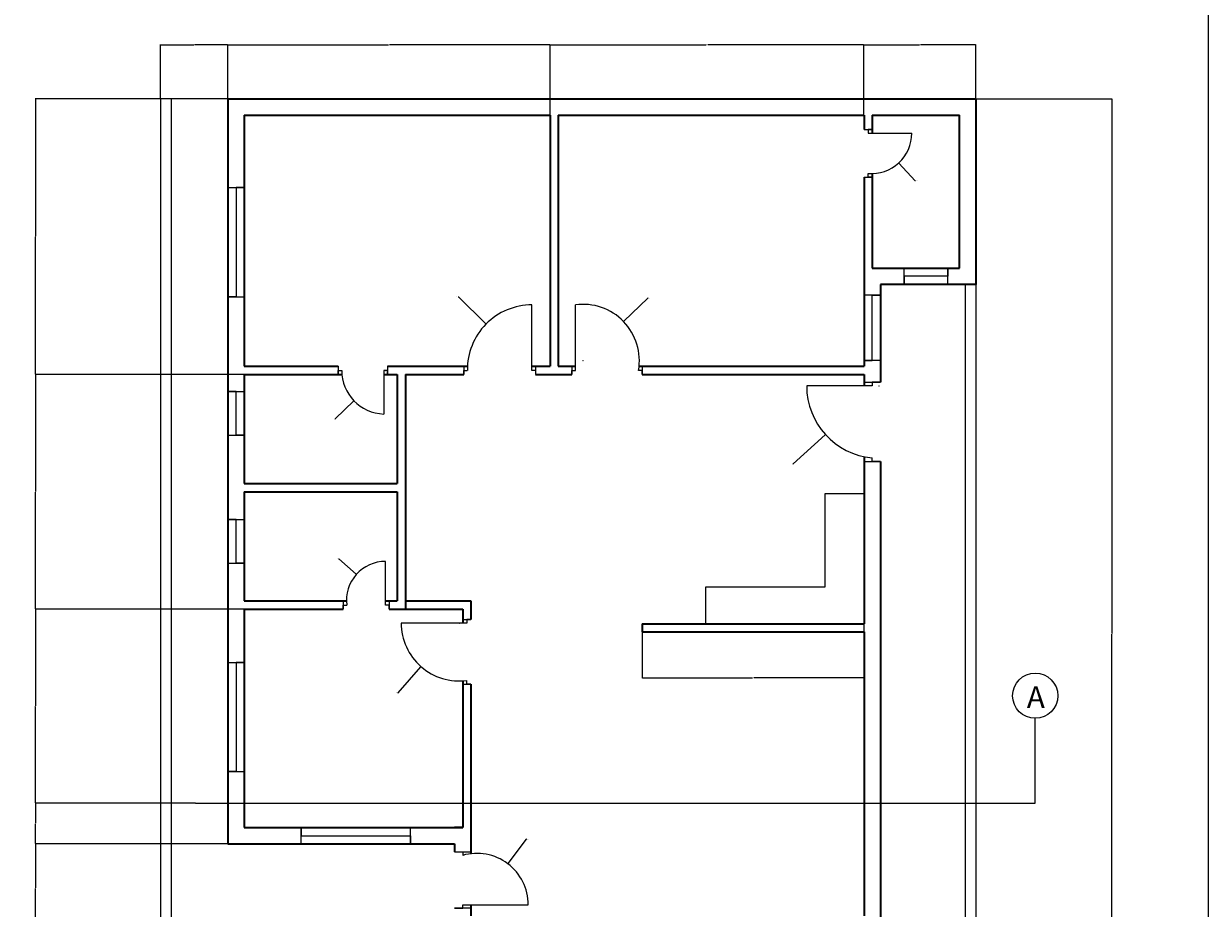
# Model space of a CAD drawing. Units: inches. Extents: x 1587 to 2880, y 1287 to 2423.
# Tile 7 of 8: x 2229 to 2880, y 1543 to 2030. Entities that reach past the tile are written whole.
import ezdxf

# ---------------------------------------------------------------- set-up
doc = ezdxf.new("R2010")
doc.units = ezdxf.units.IN
for name, color, linetype, lineweight in [('A-ANNO-DIMS', 2, 'Continuous', 18), ('A-ANNO-SYMB', 5, 'Continuous', 25), ('A-ANNO-TTLB', 7, 'Continuous', 25), ('A-DOOR', 3, 'Continuous', 18), ('A-FLOR-FIXT', 8, 'Continuous', 18), ('A-GLAZ', 4, 'Continuous', 18), ('A-WALL', 7, 'Continuous', 35), ('C-PROP', 8, 'Continuous', 25)]:
    doc.layers.add(name, color=color, linetype=linetype, lineweight=lineweight)
doc.layers.add('A-WALL-PATT', color=251, linetype='Continuous', lineweight=13, true_color=0x636466)
doc.styles.get("Standard").update_dxf_attribs({"font": 'arial.ttf'})
doc.dimstyles.get("Standard").update_dxf_attribs({"dimtxt": 0.18, "dimasz": 0.18, "dimexe": 0.18, "dimexo": 0.0625, "dimgap": 0.09, "dimtad": 0, "dimtih": 1, "dimtoh": 1, "dimdec": 4, "dimzin": 0, "dimdsep": 46, "dimtxsty": 'Standard', "dimcen": 0.09, "dimadec": 0, "dimazin": 0, "dimtfac": 1, "dimtdec": 4, "dimtofl": 0, "dimtmove": 0, "dimatfit": 3, "dimfxl": 1, "dimtolj": 1, "dimtzin": 0, "dimarcsym": 0})

# ---------------------------------------------------------------- blocks, each defined once
blk = doc.blocks.new('WIN-60IN')
for p, q in [((0, 60), (9, 60)), ((9, 60), (4.5, 60)), ((4.5, 60), (4.5, 0)), ((4.5, 0), (0, 0)), ((0, 0), (9, 0))]:
    blk.add_line(p, q)
blk = doc.blocks.new('WIN-24IN')
for p, q in [((0, 9), (0, 0)), ((24, 4.5), (24, 9)), ((24, 9), (24, 0)), ((0, 0), (0, 4.5)), ((0, 4.5), (24, 4.5))]:
    blk.add_line(p, q)
blk = doc.blocks.new('WIN-36IN')
for p, q in [((0, 36), (9, 36)), ((9, 36), (4.5, 36)), ((4.5, 36), (4.5, 0)), ((4.5, 0), (0, 0)), ((0, 0), (9, 0))]:
    blk.add_line(p, q)
blk = doc.blocks.new('DOOR-24IN-GUEST-BATH')
for p, q in [((23.33, 2.25), (23.33, 26.25)), ((0, 4.5), (0, 0)), ((0, 0), (0, 2.25)), ((0, 2.25), (2, 2.25)), ((25.33, 2.25), (23.33, 2.25)), ((25.33, 4.5), (25.33, 0)), ((25.33, 0), (25.33, 2.25))]:
    blk.add_line(p, q)
blk.add_arc((23.33, 4.77), 21.48, 90, 186.73236)
blk = doc.blocks.new('DOOR-24IN-BED1-BATH')
for p, q in [((0, 26.25), (0, 21.75)), ((27.11, 26.25), (27.11, 21.75)), ((0, 21.75), (0, 24)), ((0, 24), (2, 24)), ((27.11, 24), (25.11, 24)), ((25.11, 24), (25.11, 0)), ((27.11, 21.75), (27.11, 24))]:
    blk.add_line(p, q)
blk.add_arc((26.02, 24), 24.02, 180, 267.83008)
blk = doc.blocks.new('DOOR-36IN-BED1')
for p, q in [((37.52, 2.25), (37.52, 38.25)), ((0, 4.5), (0, 0)), ((0, 0), (0, 2.25)), ((0, 2.25), (2, 2.25)), ((39.52, 2.25), (37.52, 2.25)), ((39.52, 4.5), (39.52, 0))]:
    blk.add_line(p, q)
blk.add_arc((37.52, 2.73), 35.52, 90, 180.77456)
blk = doc.blocks.new('DOOR-36IN-BED2')
for p, q in [((2, 2.25), (2, 38.25)), ((0, 4.5), (0, 0)), ((0, 0), (0, 2.25)), ((0, 2.25), (2, 2.25)), ((38.7, 2.25), (36.7, 2.25)), ((38.7, 4.5), (38.7, 0)), ((38.7, 0), (38.7, 2.25))]:
    blk.add_line(p, q)
blk.add_arc((6.24, 7.62), 30.93, 350.00897, 97.87967)
blk = doc.blocks.new('DOOR-24IN-BED2-BATH')
for p, q in [((0, 26.03), (4.5, 26.03)), ((4.5, 26.03), (2.25, 26.03)), ((2.25, 26.03), (2.25, 24.03)), ((2.25, 24.03), (26.25, 24.03)), ((0, 0), (4.5, 0)), ((2.25, 0), (2.25, 2)), ((4.5, 0), (2.25, 0))]:
    blk.add_line(p, q)
blk.add_arc((4.13, 24.03), 22.12, 265.1111, 0)
blk = doc.blocks.new('DOOR-36IN-ENTRY')
for p, q in [((0, 31.08), (9, 31.08)), ((4.5, 31.08), (4.5, 29.08)), ((9, 0), (0, 0)), ((0, 0), (4.5, 0)), ((4.5, 0), (4.5, 2)), ((4.5, 2), (40.5, 2))]:
    blk.add_line(p, q)
blk.add_arc((12.32, 2), 28.18, 0, 106.09946)
blk = doc.blocks.new('DOOR-36IN-GUEST')
for p, q in [((36, 33.56), (0, 33.56)), ((33.75, 35.56), (38.25, 35.56)), ((38.25, 35.56), (36, 35.56)), ((36, 35.56), (36, 33.56)), ((33.75, 0), (38.25, 0)), ((36, 0), (36, 2)), ((38.25, 0), (36, 0))]:
    blk.add_line(p, q)
blk.add_arc((31.83, 33.56), 31.83, 180, 277.524)
blk = doc.blocks.new('DOOR-36IN-KITCHEN')
for p, q in [((36, 41.64), (0, 41.64)), ((31.5, 43.64), (31.5, 43.64)), ((31.5, 43.64), (40.5, 43.64)), ((40.5, 43.64), (36, 43.64)), ((36, 43.64), (36, 41.64)), ((31.5, 0), (40.5, 0)), ((36, 0), (36, 2)), ((40.5, 0), (36, 0))]:
    blk.add_line(p, q)
blk.add_arc((39.83, 41.64), 39.83, 180, 264.48319)
blk = doc.blocks.new('COUNTER-L-PLAN')
for p, q in [((65.63, 20.29), (65.63, 71.6)), ((65.63, 71.6), (86.95, 71.6)), ((0, 0), (0, 20.29)), ((0, 20.29), (65.63, 20.29))]:
    blk.add_line(p, q)
blk = doc.blocks.new('*D46')
at = {"layer": 'A-ANNO-DIMS', "color": 0, "lineweight": -2, "transparency": 16777216}
for p, q in [((2752.6, 1988.39), (2827.47, 1988.39)), ((2827.29, 1988.21), (2827.29, 1694.57)), ((2827.29, 1400.57), (2827.29, 1694.2)), ((2752.6, 1400.39), (2827.47, 1400.39))]:
    blk.add_line(p, q, dxfattribs=at)
at = {"layer": 'A-ANNO-DIMS', "color": 0, "transparency": 16777216}
for points in [[(2827.26, 1988.21), (2827.32, 1988.21), (2827.29, 1988.39)], [(2827.26, 1400.57), (2827.32, 1400.57), (2827.29, 1400.39)]]:
    blk.add_solid(points, dxfattribs=at)
at = {"layer": 'Defpoints', "color": 0, "transparency": 16777216}
for p in [(2752.53, 1988.39), (2827.29, 1988.39), (2752.53, 1400.39)]:
    blk.add_point(p, dxfattribs=at)
at = {"layer": 'A-ANNO-DIMS', "color": 0, "transparency": 16777216, "insert": (2827.29, 1694.39), "char_height": 0.18, "attachment_point": 5}
blk.add_mtext('\\A1;588', dxfattribs=at)
blk = doc.blocks.new('*D48')
at = {"layer": 'A-ANNO-DIMS', "color": 0, "lineweight": -2, "transparency": 16777216}
for p, q in [((2304.53, 1988.45), (2304.53, 2018.32)), ((2304.71, 2018.14), (2322.82, 2018.14)), ((2341.35, 2018.14), (2323.25, 2018.14)), ((2341.53, 1988.45), (2341.53, 2018.32))]:
    blk.add_line(p, q, dxfattribs=at)
at = {"layer": 'A-ANNO-DIMS', "color": 0, "transparency": 16777216}
for points in [[(2304.71, 2018.17), (2304.71, 2018.11), (2304.53, 2018.14)], [(2341.35, 2018.17), (2341.35, 2018.11), (2341.53, 2018.14)]]:
    blk.add_solid(points, dxfattribs=at)
at = {"layer": 'Defpoints', "color": 0, "transparency": 16777216}
for p in [(2341.53, 2018.14), (2304.53, 1988.39), (2341.53, 1988.39)]:
    blk.add_point(p, dxfattribs=at)
at = {"layer": 'A-ANNO-DIMS', "color": 0, "transparency": 16777216, "insert": (2323.03, 2018.14), "char_height": 0.18, "attachment_point": 5}
blk.add_mtext('\\A1;37', dxfattribs=at)
blk = doc.blocks.new('*D49')
at = {"layer": 'A-ANNO-DIMS', "color": 0, "lineweight": -2, "transparency": 16777216}
for p, q in [((2341.53, 1988.45), (2341.53, 2018.32)), ((2341.71, 2018.14), (2429.75, 2018.14)), ((2518.35, 2018.14), (2430.31, 2018.14)), ((2518.53, 1979.45), (2518.53, 2018.32))]:
    blk.add_line(p, q, dxfattribs=at)
at = {"layer": 'A-ANNO-DIMS', "color": 0, "transparency": 16777216}
for points in [[(2341.71, 2018.17), (2341.71, 2018.11), (2341.53, 2018.14)], [(2518.35, 2018.17), (2518.35, 2018.11), (2518.53, 2018.14)]]:
    blk.add_solid(points, dxfattribs=at)
at = {"layer": 'Defpoints', "color": 0, "transparency": 16777216}
for p in [(2518.53, 2018.14), (2341.53, 1988.39), (2518.53, 1979.39)]:
    blk.add_point(p, dxfattribs=at)
at = {"layer": 'A-ANNO-DIMS', "color": 0, "transparency": 16777216, "insert": (2430.03, 2018.14), "char_height": 0.18, "attachment_point": 5}
blk.add_mtext('\\A1;177', dxfattribs=at)
blk = doc.blocks.new('*D50')
at = {"layer": 'A-ANNO-DIMS', "color": 0, "lineweight": -2, "transparency": 16777216}
for p, q in [((2518.53, 1979.45), (2518.53, 2018.32)), ((2518.71, 2018.14), (2604.4, 2018.14)), ((2690.85, 2018.14), (2605.17, 2018.14)), ((2691.03, 1979.45), (2691.03, 2018.32))]:
    blk.add_line(p, q, dxfattribs=at)
at = {"layer": 'A-ANNO-DIMS', "color": 0, "transparency": 16777216}
for points in [[(2518.71, 2018.17), (2518.71, 2018.11), (2518.53, 2018.14)], [(2690.85, 2018.17), (2690.85, 2018.11), (2691.03, 2018.14)]]:
    blk.add_solid(points, dxfattribs=at)
at = {"layer": 'Defpoints', "color": 0, "transparency": 16777216}
for p in [(2691.03, 2018.14), (2518.53, 1979.39), (2691.03, 1979.39)]:
    blk.add_point(p, dxfattribs=at)
at = {"layer": 'A-ANNO-DIMS', "color": 0, "transparency": 16777216, "insert": (2604.78, 2018.14), "char_height": 0.18, "attachment_point": 5}
blk.add_mtext('\\A1;172.5', dxfattribs=at)
blk = doc.blocks.new('*D51')
at = {"layer": 'A-ANNO-DIMS', "color": 0, "lineweight": -2, "transparency": 16777216}
for p, q in [((2691.03, 1979.45), (2691.03, 2018.32)), ((2691.21, 2018.14), (2721.46, 2018.14)), ((2752.35, 2018.14), (2722.11, 2018.14)), ((2752.53, 1988.45), (2752.53, 2018.32))]:
    blk.add_line(p, q, dxfattribs=at)
at = {"layer": 'A-ANNO-DIMS', "color": 0, "transparency": 16777216}
for points in [[(2691.21, 2018.17), (2691.21, 2018.11), (2691.03, 2018.14)], [(2752.35, 2018.17), (2752.35, 2018.11), (2752.53, 2018.14)]]:
    blk.add_solid(points, dxfattribs=at)
at = {"layer": 'Defpoints', "color": 0, "transparency": 16777216}
for p in [(2752.53, 2018.14), (2752.53, 1988.39), (2691.03, 1979.39)]:
    blk.add_point(p, dxfattribs=at)
at = {"layer": 'A-ANNO-DIMS', "color": 0, "transparency": 16777216, "insert": (2721.78, 2018.14), "char_height": 0.18, "attachment_point": 5}
blk.add_mtext('\\A1;61.5', dxfattribs=at)
blk = doc.blocks.new('*D58')
at = {"layer": 'A-ANNO-DIMS', "color": 0, "lineweight": -2, "transparency": 16777216}
for p, q in [((2341.47, 1578.89), (2235.59, 1578.89)), ((2235.77, 1578.71), (2235.77, 1554.82)), ((2235.77, 1530.57), (2235.77, 1554.45)), ((2465.97, 1530.39), (2235.59, 1530.39))]:
    blk.add_line(p, q, dxfattribs=at)
at = {"layer": 'A-ANNO-DIMS', "color": 0, "transparency": 16777216}
for points in [[(2235.74, 1578.71), (2235.8, 1578.71), (2235.77, 1578.89)], [(2235.74, 1530.57), (2235.8, 1530.57), (2235.77, 1530.39)]]:
    blk.add_solid(points, dxfattribs=at)
at = {"layer": 'Defpoints', "color": 0, "transparency": 16777216}
for p in [(2235.77, 1578.89), (2341.53, 1578.89), (2466.03, 1530.39)]:
    blk.add_point(p, dxfattribs=at)
at = {"layer": 'A-ANNO-DIMS', "color": 0, "transparency": 16777216, "insert": (2235.77, 1554.64), "char_height": 0.18, "attachment_point": 5}
blk.add_mtext('\\A1;48.5', dxfattribs=at)
blk = doc.blocks.new('*D59')
at = {"layer": 'A-ANNO-DIMS', "color": 0, "lineweight": -2, "transparency": 16777216}
for p, q in [((2265.45, 1601.25), (2235.59, 1601.25)), ((2235.77, 1601.07), (2235.77, 1590.25)), ((2235.77, 1579.07), (2235.77, 1589.88)), ((2341.47, 1578.89), (2235.59, 1578.89))]:
    blk.add_line(p, q, dxfattribs=at)
at = {"layer": 'A-ANNO-DIMS', "color": 0, "transparency": 16777216}
for points in [[(2235.74, 1601.07), (2235.8, 1601.07), (2235.77, 1601.25)], [(2235.74, 1579.07), (2235.8, 1579.07), (2235.77, 1578.89)]]:
    blk.add_solid(points, dxfattribs=at)
at = {"layer": 'Defpoints', "color": 0, "transparency": 16777216}
for p in [(2235.77, 1601.25), (2265.52, 1601.25), (2341.53, 1578.89)]:
    blk.add_point(p, dxfattribs=at)
at = {"layer": 'A-ANNO-DIMS', "color": 0, "transparency": 16777216, "insert": (2235.77, 1590.07), "char_height": 0.18, "attachment_point": 5}
blk.add_mtext('\\A1;22.36', dxfattribs=at)
blk = doc.blocks.new('*D60')
at = {"layer": 'A-ANNO-DIMS', "color": 0, "lineweight": -2, "transparency": 16777216}
for p, q in [((2350.47, 1707.89), (2235.59, 1707.89)), ((2235.77, 1707.71), (2235.77, 1654.75)), ((2235.77, 1601.43), (2235.77, 1654.38)), ((2265.45, 1601.25), (2235.59, 1601.25))]:
    blk.add_line(p, q, dxfattribs=at)
at = {"layer": 'A-ANNO-DIMS', "color": 0, "transparency": 16777216}
for points in [[(2235.74, 1707.71), (2235.8, 1707.71), (2235.77, 1707.89)], [(2235.74, 1601.43), (2235.8, 1601.43), (2235.77, 1601.25)]]:
    blk.add_solid(points, dxfattribs=at)
at = {"layer": 'Defpoints', "color": 0, "transparency": 16777216}
for p in [(2235.77, 1707.89), (2350.53, 1707.89), (2265.52, 1601.25)]:
    blk.add_point(p, dxfattribs=at)
at = {"layer": 'A-ANNO-DIMS', "color": 0, "transparency": 16777216, "insert": (2235.77, 1654.57), "char_height": 0.18, "attachment_point": 5}
blk.add_mtext('\\A1;106.64', dxfattribs=at)
blk = doc.blocks.new('*D61')
at = {"layer": 'A-ANNO-DIMS', "color": 0, "lineweight": -2, "transparency": 16777216}
for p, q in [((2350.47, 1836.89), (2235.59, 1836.89)), ((2235.77, 1836.71), (2235.77, 1772.57)), ((2235.77, 1708.07), (2235.77, 1772.2)), ((2350.47, 1707.89), (2235.59, 1707.89))]:
    blk.add_line(p, q, dxfattribs=at)
at = {"layer": 'A-ANNO-DIMS', "color": 0, "transparency": 16777216}
for points in [[(2235.74, 1836.71), (2235.8, 1836.71), (2235.77, 1836.89)], [(2235.74, 1708.07), (2235.8, 1708.07), (2235.77, 1707.89)]]:
    blk.add_solid(points, dxfattribs=at)
at = {"layer": 'Defpoints', "color": 0, "transparency": 16777216}
for p in [(2235.77, 1836.89), (2350.53, 1836.89), (2350.53, 1707.89)]:
    blk.add_point(p, dxfattribs=at)
at = {"layer": 'A-ANNO-DIMS', "color": 0, "transparency": 16777216, "insert": (2235.77, 1772.39), "char_height": 0.18, "attachment_point": 5}
blk.add_mtext('\\A1;129', dxfattribs=at)
blk = doc.blocks.new('*D62')
at = {"layer": 'A-ANNO-DIMS', "color": 0, "lineweight": -2, "transparency": 16777216}
for p, q in [((2341.47, 1988.39), (2235.59, 1988.39)), ((2235.77, 1988.21), (2235.77, 1912.82)), ((2235.77, 1837.07), (2235.77, 1912.45)), ((2350.47, 1836.89), (2235.59, 1836.89))]:
    blk.add_line(p, q, dxfattribs=at)
at = {"layer": 'A-ANNO-DIMS', "color": 0, "transparency": 16777216}
for points in [[(2235.74, 1988.21), (2235.8, 1988.21), (2235.77, 1988.39)], [(2235.74, 1837.07), (2235.8, 1837.07), (2235.77, 1836.89)]]:
    blk.add_solid(points, dxfattribs=at)
at = {"layer": 'Defpoints', "color": 0, "transparency": 16777216}
for p in [(2235.77, 1988.39), (2341.53, 1988.39), (2350.53, 1836.89)]:
    blk.add_point(p, dxfattribs=at)
at = {"layer": 'A-ANNO-DIMS', "color": 0, "transparency": 16777216, "insert": (2235.77, 1912.64), "char_height": 0.18, "attachment_point": 5}
blk.add_mtext('\\A1;151.5', dxfattribs=at)
blk = doc.blocks.new('*D81')
at = {"layer": 'A-ANNO-DIMS', "color": 0, "lineweight": -2, "transparency": 16777216}
for p, q in [((2569.14, 1699.82), (2569.14, 1669.96)), ((2691.03, 1699.82), (2691.03, 1669.96)), ((2569.32, 1670.14), (2629.7, 1670.14)), ((2690.85, 1670.14), (2630.47, 1670.14))]:
    blk.add_line(p, q, dxfattribs=at)
at = {"layer": 'A-ANNO-DIMS', "color": 0, "transparency": 16777216}
for points in [[(2569.32, 1670.17), (2569.32, 1670.11), (2569.14, 1670.14)], [(2690.85, 1670.17), (2690.85, 1670.11), (2691.03, 1670.14)]]:
    blk.add_solid(points, dxfattribs=at)
at = {"layer": 'Defpoints', "color": 0, "transparency": 16777216}
for p in [(2569.14, 1699.89), (2691.03, 1699.89), (2569.14, 1670.14)]:
    blk.add_point(p, dxfattribs=at)
at = {"layer": 'A-ANNO-DIMS', "color": 0, "transparency": 16777216, "insert": (2630.09, 1670.14), "char_height": 0.18, "attachment_point": 5}
blk.add_mtext('\\A1;121.9', dxfattribs=at)
blk = doc.blocks.new('*D100')
at = {"layer": 'A-ANNO-DIMS', "color": 0, "lineweight": -2, "transparency": 16777216}
for p, q in [((2699.27, 1830.63), (2699.45, 1830.63)), ((2699.36, 1830.54), (2699.36, 1830.72)), ((2652.18, 1787.79), (2669.74, 1803.74)), ((2652, 1787.79), (2652.18, 1787.79))]:
    blk.add_line(p, q, dxfattribs=at)
at = {"layer": 'A-ANNO-DIMS', "color": 0, "transparency": 16777216}
blk.add_solid([(2669.72, 1803.76), (2669.76, 1803.71), (2669.88, 1803.86)], dxfattribs=at)
at = {"layer": 'Defpoints', "color": 0, "transparency": 16777216}
for p in [(2699.36, 1830.63), (2669.88, 1803.86)]:
    blk.add_point(p, dxfattribs=at)
at = {"layer": 'A-ANNO-DIMS', "color": 0, "transparency": 16777216, "insert": (2651.53, 1787.79), "char_height": 0.18, "attachment_point": 5}
blk.add_mtext('\\A1;R39.83', dxfattribs=at)
blk = doc.blocks.new('*D101')
at = {"layer": 'A-ANNO-DIMS', "color": 0, "lineweight": -2, "transparency": 16777216}
for p, q in [((2467.97, 1879.53), (2468.15, 1879.53)), ((2468.15, 1879.53), (2483.2, 1864.69)), ((2508.52, 1839.62), (2508.7, 1839.62)), ((2508.61, 1839.53), (2508.61, 1839.71))]:
    blk.add_line(p, q, dxfattribs=at)
at = {"layer": 'A-ANNO-DIMS', "color": 0, "transparency": 16777216}
blk.add_solid([(2483.22, 1864.71), (2483.17, 1864.67), (2483.32, 1864.56)], dxfattribs=at)
at = {"layer": 'Defpoints', "color": 0, "transparency": 16777216}
for p in [(2483.32, 1864.56), (2508.61, 1839.62)]:
    blk.add_point(p, dxfattribs=at)
at = {"layer": 'A-ANNO-DIMS', "color": 0, "transparency": 16777216, "insert": (2467.49, 1879.53), "char_height": 0.18, "attachment_point": 5}
blk.add_mtext('\\A1;R35.52', dxfattribs=at)
blk = doc.blocks.new('*D102')
at = {"layer": 'A-ANNO-DIMS', "color": 0, "lineweight": -2, "transparency": 16777216}
for p, q in [((2468.53, 1700.27), (2468.71, 1700.27)), ((2468.62, 1700.18), (2468.62, 1700.36)), ((2435.04, 1661.97), (2447.51, 1676.2)), ((2434.86, 1661.97), (2435.04, 1661.97))]:
    blk.add_line(p, q, dxfattribs=at)
at = {"layer": 'A-ANNO-DIMS', "color": 0, "transparency": 16777216}
blk.add_solid([(2447.49, 1676.22), (2447.54, 1676.18), (2447.63, 1676.33)], dxfattribs=at)
at = {"layer": 'Defpoints', "color": 0, "transparency": 16777216}
for p in [(2468.62, 1700.27), (2447.63, 1676.33)]:
    blk.add_point(p, dxfattribs=at)
at = {"layer": 'A-ANNO-DIMS', "color": 0, "transparency": 16777216, "insert": (2434.38, 1661.97), "char_height": 0.18, "attachment_point": 5}
blk.add_mtext('\\A1;R31.83', dxfattribs=at)
blk = doc.blocks.new('*D103')
at = {"layer": 'A-ANNO-DIMS', "color": 0, "lineweight": -2, "transparency": 16777216}
for p, q in [((2572.32, 1878.84), (2559.08, 1866.09)), ((2572.5, 1878.84), (2572.32, 1878.84)), ((2536.6, 1844.5), (2536.78, 1844.5)), ((2536.69, 1844.41), (2536.69, 1844.59))]:
    blk.add_line(p, q, dxfattribs=at)
at = {"layer": 'A-ANNO-DIMS', "color": 0, "transparency": 16777216}
blk.add_solid([(2559.06, 1866.11), (2559.11, 1866.07), (2558.96, 1865.96)], dxfattribs=at)
at = {"layer": 'Defpoints', "color": 0, "transparency": 16777216}
for p in [(2558.96, 1865.96), (2536.69, 1844.5)]:
    blk.add_point(p, dxfattribs=at)
at = {"layer": 'A-ANNO-DIMS', "color": 0, "transparency": 16777216, "insert": (2573.05, 1878.84), "char_height": 0.18, "attachment_point": 5}
blk.add_mtext('\\A1;R30.926', dxfattribs=at)
blk = doc.blocks.new('*D104')
at = {"layer": 'A-ANNO-DIMS', "color": 0, "lineweight": -2, "transparency": 16777216}
for p, q in [((2505.46, 1581.52), (2495.4, 1568.15)), ((2505.64, 1581.52), (2505.46, 1581.52)), ((2478.26, 1545.48), (2478.44, 1545.48)), ((2478.35, 1545.39), (2478.35, 1545.57))]:
    blk.add_line(p, q, dxfattribs=at)
at = {"layer": 'A-ANNO-DIMS', "color": 0, "transparency": 16777216}
blk.add_solid([(2495.38, 1568.16), (2495.42, 1568.13), (2495.29, 1568)], dxfattribs=at)
at = {"layer": 'Defpoints', "color": 0, "transparency": 16777216}
for p in [(2495.29, 1568), (2478.35, 1545.48)]:
    blk.add_point(p, dxfattribs=at)
at = {"layer": 'A-ANNO-DIMS', "color": 0, "transparency": 16777216, "insert": (2506.19, 1581.52), "char_height": 0.18, "attachment_point": 5}
blk.add_mtext('\\A1;R28.184', dxfattribs=at)
blk = doc.blocks.new('*D105')
at = {"layer": 'A-ANNO-DIMS', "color": 0, "lineweight": -2, "transparency": 16777216}
for p, q in [((2428.01, 1839.14), (2428.19, 1839.14)), ((2428.1, 1839.05), (2428.1, 1839.23)), ((2400.42, 1812.48), (2410.67, 1822.35)), ((2400.24, 1812.48), (2400.42, 1812.48))]:
    blk.add_line(p, q, dxfattribs=at)
at = {"layer": 'A-ANNO-DIMS', "color": 0, "transparency": 16777216}
blk.add_solid([(2410.65, 1822.38), (2410.69, 1822.33), (2410.8, 1822.48)], dxfattribs=at)
at = {"layer": 'Defpoints', "color": 0, "transparency": 16777216}
for p in [(2428.1, 1839.14), (2410.8, 1822.48)]:
    blk.add_point(p, dxfattribs=at)
at = {"layer": 'A-ANNO-DIMS', "color": 0, "transparency": 16777216, "insert": (2399.69, 1812.48), "char_height": 0.18, "attachment_point": 5}
blk.add_mtext('\\A1;R24.017', dxfattribs=at)
blk = doc.blocks.new('*D106')
at = {"layer": 'A-ANNO-DIMS', "color": 0, "lineweight": -2, "transparency": 16777216}
for p, q in [((2695.08, 1969.44), (2695.26, 1969.44)), ((2695.17, 1969.35), (2695.17, 1969.53)), ((2719.1, 1943.37), (2710.25, 1953.02)), ((2719.28, 1943.37), (2719.1, 1943.37))]:
    blk.add_line(p, q, dxfattribs=at)
at = {"layer": 'A-ANNO-DIMS', "color": 0, "transparency": 16777216}
blk.add_solid([(2710.27, 1953.04), (2710.22, 1953), (2710.13, 1953.15)], dxfattribs=at)
at = {"layer": 'Defpoints', "color": 0, "transparency": 16777216}
for p in [(2695.17, 1969.44), (2710.13, 1953.15)]:
    blk.add_point(p, dxfattribs=at)
at = {"layer": 'A-ANNO-DIMS', "color": 0, "transparency": 16777216, "insert": (2719.83, 1943.37), "char_height": 0.18, "attachment_point": 5}
blk.add_mtext('\\A1;R22.115', dxfattribs=at)
blk = doc.blocks.new('*D107')
at = {"layer": 'A-ANNO-DIMS', "color": 0, "lineweight": -2, "transparency": 16777216}
for p, q in [((2402.28, 1735.49), (2402.46, 1735.49)), ((2402.46, 1735.49), (2411.96, 1727.05)), ((2428.06, 1712.66), (2428.24, 1712.66)), ((2428.15, 1712.57), (2428.15, 1712.75))]:
    blk.add_line(p, q, dxfattribs=at)
at = {"layer": 'A-ANNO-DIMS', "color": 0, "transparency": 16777216}
blk.add_solid([(2411.98, 1727.07), (2411.94, 1727.02), (2412.09, 1726.93)], dxfattribs=at)
at = {"layer": 'Defpoints', "color": 0, "transparency": 16777216}
for p in [(2412.09, 1726.93), (2428.15, 1712.66)]:
    blk.add_point(p, dxfattribs=at)
at = {"layer": 'A-ANNO-DIMS', "color": 0, "transparency": 16777216, "insert": (2401.8, 1735.49), "char_height": 0.18, "attachment_point": 5}
blk.add_mtext('\\A1;R21.48', dxfattribs=at)

msp = doc.modelspace()

# ---------------------------------------------------------------- hatches: boundary and pattern name
at = {"layer": 'A-WALL-PATT'}
h = msp.add_hatch(color=256, dxfattribs=at)
h.dxf.hatch_style = 1
h.paths.add_polyline_path([(2190.3423, 1988.3868), (2181.3423, 1988.3868), (2137.8423, 1988.3868), (1779.3423, 1988.3868), (1779.3423, 1939.6287), (1788.3423, 1939.6287), (1788.3423, 1979.3868), (1956.3423, 1979.3868), (1956.3423, 1841.3868), (1948.4175, 1841.3868), (1948.4175, 1836.8868), (1968.256, 1836.8868), (1968.256, 1839.1368), (1968.256, 1841.3868), (1960.8423, 1841.3868), (1960.8423, 1979.3868), (2128.8423, 1979.3868), (2128.8423, 1971.4394), (2133.3423, 1971.4394), (2133.3423, 1979.3868), (2181.3423, 1979.3868), (2181.3423, 1895.3868), (2174.9842, 1895.3868), (2174.9842, 1886.3868), (2190.3423, 1886.3868), (2190.3423, 1895.3868)])
h.paths.add_polyline_path([(1788.3423, 1879.6287), (1779.3423, 1879.6287), (1779.3423, 1827.4437), (1788.3423, 1827.4437), (1788.3423, 1836.8868), (1839.8915, 1836.8868), (1839.8915, 1839.1368), (1839.8915, 1841.3868), (1788.3423, 1841.3868)])
h.paths.add_polyline_path([(1876.8423, 1836.8868), (1908.901, 1836.8868), (1908.901, 1839.1368), (1908.901, 1841.3868), (1866.9993, 1841.3868), (1866.9993, 1836.8868), (1872.3423, 1836.8868), (1872.3423, 1776.8868), (1788.3423, 1776.8868), (1788.3423, 1803.4437), (1779.3423, 1803.4437), (1779.3423, 1757.1447), (1788.3423, 1757.1447), (1788.3423, 1772.3868), (1872.3423, 1772.3868), (1872.3423, 1712.3868), (1867.9542, 1712.3868), (1867.9542, 1707.8868), (1876.8423, 1707.8868), (1876.8423, 1772.3868)])
h.paths.add_polyline_path([(1842.6206, 1710.1368), (1842.6206, 1712.3868), (1788.3423, 1712.3868), (1788.3423, 1733.1447), (1779.3423, 1733.1447), (1779.3423, 1678.6557), (1788.3423, 1678.6557), (1788.3423, 1707.8868), (1842.6206, 1707.8868)])
h.paths.add_polyline_path([(1912.8423, 1712.3868), (1908.3423, 1712.3868), (1876.8423, 1712.3868), (1876.8423, 1707.8868), (1908.3423, 1707.8868), (1908.3423, 1702.2679), (1912.8423, 1702.2679)])
h.paths.add_polyline_path([(2137.8423, 1844.5168), (2128.8423, 1844.5168), (2128.8423, 1841.3868), (2006.9533, 1841.3868), (2006.9533, 1836.8868), (2128.8423, 1836.8868), (2128.8423, 1832.632), (2137.8423, 1832.632)])
h.paths.add_polyline_path([(1997.6598, 1534.8868), (1997.6598, 1539.3868), (1912.8423, 1539.3868), (1912.8423, 1543.4794), (1903.8423, 1543.4794), (1903.8423, 1530.3868), (1997.6598, 1530.3868)])
h.paths.add_polyline_path([(1912.8423, 1666.7101), (1910.5923, 1666.7101), (1908.3423, 1666.7101), (1908.3423, 1587.8868), (1903.8423, 1587.8868), (1879.6624, 1587.8868), (1879.6624, 1578.8868), (1903.8423, 1578.8868), (1903.8423, 1574.5584), (1912.8423, 1574.5584), (1912.8423, 1578.8868), (1912.8423, 1587.8868)])
h.paths.add_polyline_path([(1788.3423, 1618.6557), (1779.3423, 1618.6557), (1779.3423, 1578.8868), (1819.6624, 1578.8868), (1819.6624, 1583.3868), (1819.6624, 1587.8868), (1788.3423, 1587.8868)])
h.paths.add_polyline_path([(2133.3423, 1945.4046), (2131.0923, 1945.4046), (2128.8423, 1945.4046), (2128.8423, 1880.5168), (2137.8423, 1880.5168), (2137.8423, 1886.3868), (2150.9842, 1886.3868), (2150.9842, 1890.8868), (2150.9842, 1895.3868), (2133.3423, 1895.3868)], flags=17)
h.paths.add_polyline_path([(2137.8423, 1788.9874), (2133.3423, 1788.9874), (2128.8423, 1788.9874), (2128.8423, 1699.8868), (2006.9533, 1699.8868), (2006.9533, 1695.3868), (2128.8423, 1695.3868), (2128.8423, 1539.3868), (2057.6598, 1539.3868), (2057.6598, 1530.3868), (2128.8423, 1530.3868), (2128.8423, 1461.3868), (1988.2941, 1461.3868), (1988.2941, 1452.3868), (2137.8423, 1452.3868), (2137.8423, 1530.3868)])
h.paths.add_polyline_path([(1866.9166, 1348.94), (2042.3313, 1348.94), (2042.3313, 1371.6078), (1866.9166, 1371.6078)], flags=9)
h.paths.add_polyline_path([(2758.0473, 2126.4845), (2848.522, 2126.4845), (2848.522, 2138.8487), (2758.0473, 2138.8487)], flags=9)
h.paths.add_polyline_path([(2742.9428, 2216.0014), (2782.483, 2216.0014), (2782.483, 2228.3657), (2742.9428, 2228.3657)], flags=9)
h.paths.add_polyline_path([(2749.234, 2261.9992), (2784.0963, 2261.9992), (2784.0963, 2274.3634), (2749.234, 2274.3634)], flags=9)
h.paths.add_polyline_path([(2733.8012, 2281.8262), (2817.7726, 2281.8262), (2817.7726, 2294.1904), (2733.8012, 2294.1904)], flags=9)
h.paths.add_polyline_path([(2422.857, 2073.081), (2531.34, 2073.081), (2531.34, 2097.8095), (2422.857, 2097.8095)], flags=9)
h.paths.add_polyline_path([(1856.7732, 2082.3109), (1956.866, 2082.3109), (1956.866, 2107.0394), (1856.7732, 2107.0394)], flags=9)
h.paths.add_polyline_path([(2777.4581, 1646.9437), (2794.6887, 1646.9437), (2794.6887, 1671.6723), (2777.4581, 1671.6723)], flags=9)
h.paths.add_polyline_path([(2585.5416, 1728.5169), (2655.2006, 1728.5169), (2655.2006, 1760.9057), (2585.5416, 1760.9057)], flags=9)
h.paths.add_polyline_path([(2554.1301, 1617.6432), (2608.2079, 1617.6432), (2608.2079, 1640.032), (2554.1301, 1640.032)], flags=9)
h.paths.add_polyline_path([(2359.8658, 1678.1191), (2437.8454, 1678.1191), (2437.8454, 1700.5079), (2359.8658, 1700.5079)], flags=9)
h.paths.add_polyline_path([(2392.0171, 1749.26), (2422.3411, 1749.26), (2422.3411, 1767.9173), (2392.0171, 1767.9173)], flags=9)
h.paths.add_polyline_path([(2391.9937, 1787.5799), (2422.3177, 1787.5799), (2422.3177, 1806.2373), (2391.9937, 1806.2373)], flags=9)
h.paths.add_polyline_path([(2707.7632, 1927.6903), (2738.1623, 1927.6903), (2738.1623, 1946.3477), (2707.7632, 1946.3477)], flags=9)
h.paths.add_polyline_path([(2581.5534, 1846.9887), (2635.6148, 1846.9887), (2635.6148, 1869.3775), (2581.5534, 1869.3775)], flags=9)
h.paths.add_polyline_path([(2382.3802, 1864.4978), (2436.4416, 1864.4978), (2436.4416, 1886.8866), (2382.3802, 1886.8866)], flags=9)
h.paths.add_polyline_path([(2023.35, 1728.5169), (2093.0089, 1728.5169), (2093.0089, 1760.9057), (2023.35, 1760.9057)], flags=25)
h.paths.add_polyline_path([(1991.9385, 1617.6432), (2046.0162, 1617.6432), (2046.0162, 1640.032), (1991.9385, 1640.032)], flags=25)
h.paths.add_polyline_path([(1791.1103, 1678.1191), (1869.0899, 1678.1191), (1869.0899, 1700.5079), (1791.1103, 1700.5079)], flags=9)
h.paths.add_polyline_path([(1829.8255, 1749.26), (1860.1495, 1749.26), (1860.1495, 1767.9173), (1829.8255, 1767.9173)], flags=25)
h.paths.add_polyline_path([(1829.8021, 1787.5799), (1860.1261, 1787.5799), (1860.1261, 1806.2373), (1829.8021, 1806.2373)], flags=25)
h.paths.add_polyline_path([(2145.5716, 1927.6903), (2175.9706, 1927.6903), (2175.9706, 1946.3477), (2145.5716, 1946.3477)], flags=25)
h.paths.add_polyline_path([(2019.3617, 1846.9887), (2073.4231, 1846.9887), (2073.4231, 1869.3775), (2019.3617, 1869.3775)], flags=25)
h.paths.add_polyline_path([(1820.1886, 1864.4978), (1874.25, 1864.4978), (1874.25, 1886.8866), (1820.1886, 1886.8866)], flags=25)

# ---------------------------------------------------------------- linework, layer by layer
at = {"layer": 'A-ANNO-SYMB'}
for p, q in [((2785.1198, 1601.2461), (2785.1198, 1647.901)), ((2323.7941, 1601.2461), (2265.516, 1601.2461)), ((2323.7941, 1601.2461), (2785.1198, 1601.2461))]:
    msp.add_line(p, q, dxfattribs=at)
msp.add_circle((2785.1198, 1660.3223), 12.4213, dxfattribs=at)
at = {"layer": 'A-ANNO-TTLB'}
msp.add_lwpolyline([(1586.5185, 2423.1539), (2880.2062, 2423.1539), (2880.2062, 1286.9347), (1586.5185, 1286.9347)], close=True, dxfattribs=at)
at = {"layer": 'A-WALL'}
for p, q in [((2341.534, 1988.3868), (2341.534, 1578.8868)), ((2341.534, 1988.3868), (2341.534, 1578.8868)), ((2341.534, 1988.3868), (2700.034, 1988.3868)), ((2691.034, 1988.3868), (2695.534, 1988.3868)), ((2700.034, 1988.3868), (2748.034, 1988.3868)), ((2743.534, 1988.3868), (2752.534, 1988.3868)), ((2752.534, 1988.3868), (2752.534, 1895.3868)), ((2350.534, 1979.3868), (2350.534, 1841.3868)), ((2350.534, 1979.3868), (2518.534, 1979.3868)), ((2518.534, 1979.3868), (2518.534, 1841.3868)), ((2523.034, 1979.3868), (2523.034, 1841.3868)), ((2523.034, 1979.3868), (2691.034, 1979.3868)), ((2691.034, 1979.3868), (2691.034, 1971.4394)), ((2695.534, 1979.3868), (2695.534, 1969.4394)), ((2695.534, 1979.3868), (2743.534, 1979.3868)), ((2743.534, 1895.3868), (2743.534, 1979.3868)), ((2695.534, 1947.3272), (2695.534, 1895.3868)), ((2691.034, 1945.4046), (2691.034, 1841.3868)), ((2695.534, 1895.3868), (2743.534, 1895.3868)), ((2752.534, 1895.3868), (2752.534, 1886.3868)), ((2700.034, 1886.3868), (2700.034, 1832.632)), ((2752.534, 1886.3868), (2700.034, 1886.3868)), ((2350.534, 1841.3868), (2402.0831, 1841.3868)), ((2350.534, 1836.8868), (2350.534, 1776.8868)), ((2350.534, 1836.8868), (2404.1888, 1836.8868)), ((2427.191, 1836.8868), (2434.534, 1836.8868)), ((2429.191, 1841.3868), (2473.1335, 1841.3868)), ((2434.534, 1836.8868), (2434.534, 1776.8868)), ((2439.034, 1836.8868), (2439.034, 1772.3868)), ((2439.034, 1836.8868), (2471.0926, 1836.8868)), ((2508.6092, 1841.3868), (2518.534, 1841.3868)), ((2510.6092, 1836.8868), (2530.4477, 1836.8868)), ((2523.034, 1841.3868), (2532.4477, 1841.3868)), ((2567.4566, 1841.3868), (2691.034, 1841.3868)), ((2569.145, 1836.8868), (2691.034, 1836.8868)), ((2691.034, 1836.8868), (2691.034, 1830.632)), ((2691.034, 1791.6836), (2691.034, 1699.8868)), ((2700.034, 1788.9874), (2700.034, 1530.3868)), ((2350.534, 1776.8868), (2434.534, 1776.8868)), ((2350.534, 1772.3868), (2350.534, 1712.3868)), ((2350.534, 1772.3868), (2434.534, 1772.3868)), ((2434.534, 1772.3868), (2434.534, 1712.3868)), ((2439.034, 1772.3868), (2439.034, 1707.8868)), ((2350.534, 1712.3868), (2406.6659, 1712.3868)), ((2428.1458, 1712.3868), (2434.534, 1712.3868)), ((2439.034, 1712.3868), (2470.534, 1712.3868)), ((2470.534, 1712.3868), (2475.034, 1712.3868)), ((2475.034, 1712.3868), (2475.034, 1702.2679)), ((2350.534, 1707.8868), (2350.534, 1587.8868)), ((2350.534, 1707.8868), (2404.8123, 1707.8868)), ((2350.534, 1707.8868), (2404.8123, 1707.8868)), ((2430.1458, 1707.8868), (2439.034, 1707.8868)), ((2430.1458, 1707.8868), (2470.534, 1707.8868)), ((2470.534, 1707.8868), (2470.534, 1700.2679)), ((2569.145, 1699.8868), (2691.034, 1699.8868)), ((2569.145, 1699.8868), (2569.145, 1695.3868)), ((2569.145, 1695.3868), (2691.034, 1695.3868)), ((2691.034, 1695.3868), (2691.034, 1539.3868)), ((2470.534, 1668.4939), (2470.534, 1587.8868)), ((2475.034, 1666.7101), (2475.034, 1587.8868)), ((2350.534, 1587.8868), (2470.534, 1587.8868)), ((2470.534, 1587.8868), (2466.034, 1587.8868)), ((2475.034, 1587.8868), (2475.034, 1578.8868)), ((2341.534, 1578.8868), (2466.034, 1578.8868)), ((2466.034, 1578.8868), (2466.034, 1574.5584)), ((2475.034, 1578.8868), (2475.034, 1573.468)), ((2475.034, 1545.4794), (2475.034, 1539.3868))]:
    msp.add_line(p, q, dxfattribs=at)
at = {"layer": 'C-PROP'}
for p, q in [((2341.534, 1988.3868), (2304.534, 1988.3868)), ((2304.534, 1988.3868), (2304.534, 1400.3868)), ((2310.534, 1406.3868), (2310.534, 1988.3868)), ((2752.534, 1886.3868), (2746.534, 1886.3868)), ((2746.534, 1886.3868), (2746.534, 1406.3868)), ((2752.534, 1886.3868), (2752.534, 1400.3868))]:
    msp.add_line(p, q, dxfattribs=at)

# ---------------------------------------------------------------- block references
at = {"layer": 'A-DOOR'}
for name, p in [('DOOR-24IN-BED2-BATH', (2691.034, 1945.4046)), ('DOOR-36IN-BED1', (2471.0926, 1836.8868)), ('DOOR-36IN-BED2', (2530.4477, 1836.8868)), ('DOOR-24IN-BED1-BATH', (2402.0831, 1815.1368)), ('DOOR-36IN-KITCHEN', (2659.534, 1788.9874)), ('DOOR-24IN-GUEST-BATH', (2404.8123, 1707.8868)), ('DOOR-36IN-GUEST', (2436.784, 1666.7101)), ('DOOR-36IN-ENTRY', (2466.034, 1543.4794))]:
    msp.add_blockref(name, p, dxfattribs=at)
at = {"layer": 'A-FLOR-FIXT'}
msp.add_blockref('COUNTER-L-PLAN', (2604.0837, 1699.8868), dxfattribs=at)
at = {"layer": 'A-GLAZ'}
for p in [(2341.5337, 1879.629), (2341.5337, 1618.6559)]:
    msp.add_blockref('WIN-60IN', p, dxfattribs=at)
for name, p, rotation in [('WIN-24IN', (2737.1761, 1895.3867), 180), ('WIN-36IN', (2700.0343, 1880.5165), 180), ('WIN-24IN', (2350.5338, 1803.4434), 90.00000000000024), ('WIN-24IN', (2350.5338, 1733.1445), 90.0000000000006), ('WIN-60IN', (2441.8538, 1578.8865), 90.00000000000138)]:
    msp.add_blockref(name, p, dxfattribs=dict(at, rotation=rotation))

# ---------------------------------------------------------------- texts
at = {"layer": 'A-ANNO-SYMB', "insert": (2780.4827, 1665.4963), "char_height": 12, "attachment_point": 1}
msp.add_mtext_dynamic_manual_height_columns('A', width=34.943833, gutter_width=12.5, heights=[0], dxfattribs=at)

# ---------------------------------------------------------------- dimensions: what is measured, and where the dimension line sits
at = {"layer": 'A-ANNO-DIMS'}
for base, p1, p2, override, picture, middle in [((2341.534, 2018.1368), (2304.534, 1988.3868), (2341.534, 1988.3868), {"dimdec": 0, "dimlfac": 1, "dimrnd": 0, "dimzin": 0, "dimdsep": 46, "dimlunit": 2}, '*D48', (2323.034, 2018.1368)), ((2518.534, 2018.1368), (2341.534, 1988.3868), (2518.534, 1979.3868), {"dimdec": 0, "dimlfac": 1, "dimrnd": 0, "dimzin": 0, "dimdsep": 46, "dimlunit": 2}, '*D49', (2430.034, 2018.1368)), ((2691.034, 2018.1368), (2518.534, 1979.3868), (2691.034, 1979.3868), {"dimdec": 1, "dimlfac": 1, "dimrnd": 0, "dimzin": 0, "dimdsep": 46, "dimlunit": 2}, '*D50', (2604.784, 2018.1368)), ((2752.534, 2018.1368), (2691.034, 1979.3868), (2752.534, 1988.3868), {"dimdec": 1, "dimlfac": 1, "dimrnd": 0, "dimzin": 0, "dimdsep": 46, "dimlunit": 2}, '*D51', (2721.784, 2018.1368))]:
    dim = msp.add_linear_dim(base=base, p1=p1, p2=p2, dimstyle='Standard', override=override, dxfattribs=at)
    dim.commit()
    dim.dimension.update_dxf_attribs({"geometry": picture, "text_midpoint": middle})
for base, p1, p2, angle, override, picture, middle in [((2235.766, 1988.3868), (2350.534, 1836.8868), (2341.534, 1988.3868), 90, {"dimdec": 1, "dimlfac": 1, "dimrnd": 0, "dimzin": 0, "dimdsep": 46, "dimlunit": 2}, '*D62', (2235.766, 1912.6368)), ((2827.2911, 1988.3868), (2752.534, 1400.3868), (2752.534, 1988.3868), 90, {"dimdec": 0, "dimlfac": 1, "dimrnd": 0, "dimzin": 0, "dimdsep": 46, "dimlunit": 2}, '*D46', (2827.2911, 1694.3868)), ((2235.766, 1836.8868), (2350.534, 1707.8868), (2350.534, 1836.8868), 90, {"dimdec": 0, "dimlfac": 1, "dimrnd": 0, "dimzin": 0, "dimdsep": 46, "dimlunit": 2}, '*D61', (2235.766, 1772.3868)), ((2235.766, 1707.8868), (2265.516, 1601.2461), (2350.534, 1707.8868), 90, {"dimdec": 2, "dimlfac": 1, "dimrnd": 0, "dimzin": 0, "dimdsep": 46, "dimlunit": 2}, '*D60', (2235.766, 1654.5665)), ((2569.145, 1670.1368), (2691.034, 1699.8868), (2569.145, 1699.8868), 180, {"dimdec": 1, "dimlfac": 1, "dimrnd": 0, "dimzin": 0, "dimdsep": 46, "dimlunit": 2}, '*D81', (2630.0895, 1670.1368)), ((2235.766, 1601.2461), (2341.534, 1578.8868), (2265.516, 1601.2461), 90, {"dimdec": 2, "dimlfac": 1, "dimrnd": 0, "dimzin": 0, "dimdsep": 46, "dimlunit": 2}, '*D59', (2235.766, 1590.0665)), ((2235.766, 1578.8868), (2466.034, 1530.3868), (2341.534, 1578.8868), 90, {"dimdec": 1, "dimlfac": 1, "dimrnd": 0, "dimzin": 0, "dimdsep": 46, "dimlunit": 2}, '*D58', (2235.766, 1554.6368))]:
    dim = msp.add_linear_dim(base=base, p1=p1, p2=p2, angle=angle, dimstyle='Standard', override=override, dxfattribs=at)
    dim.commit()
    dim.dimension.update_dxf_attribs({"geometry": picture, "text_midpoint": middle})
for center, mpoint, override, picture, middle in [((2695.1687, 1969.4394), (2710.1253, 1953.1487), {"dimdec": 3, "dimlfac": 1, "dimrnd": 0, "dimzin": 0, "dimdsep": 46, "dimlunit": 2}, '*D106', (2719.8296, 1943.3743)), ((2508.6092, 1839.617), (2483.3239, 1864.5631), {"dimdec": 2, "dimlfac": 1, "dimrnd": 0, "dimzin": 0, "dimdsep": 46, "dimlunit": 2}, '*D101', (2467.4937, 1879.5308)), ((2536.6875, 1844.5024), (2558.955, 1865.964), {"dimdec": 3, "dimlfac": 1, "dimrnd": 0, "dimzin": 0, "dimdsep": 46, "dimlunit": 2}, '*D103', (2573.0452, 1878.841)), ((2428.1004, 1839.1368), (2410.7989, 1822.4789), {"dimdec": 3, "dimlfac": 1, "dimrnd": 0, "dimzin": 0, "dimdsep": 46, "dimlunit": 2}, '*D105', (2399.6883, 1812.4842)), ((2699.3631, 1830.632), (2669.8768, 1803.8568), {"dimdec": 2, "dimlfac": 1, "dimrnd": 0, "dimzin": 0, "dimdsep": 46, "dimlunit": 2}, '*D100', (2651.5251, 1787.7916)), ((2428.1458, 1712.6552), (2412.0902, 1726.9268), {"dimdec": 2, "dimlfac": 1, "dimrnd": 0, "dimzin": 0, "dimdsep": 46, "dimlunit": 2}, '*D107', (2401.7968, 1735.4898)), ((2468.6159, 1700.2679), (2447.6329, 1676.3309), {"dimdec": 2, "dimlfac": 1, "dimrnd": 0, "dimzin": 0, "dimdsep": 46, "dimlunit": 2}, '*D102', (2434.3832, 1661.9686)), ((2478.3497, 1545.4794), (2495.292, 1568.003), {"dimdec": 3, "dimlfac": 1, "dimrnd": 0, "dimzin": 0, "dimdsep": 46, "dimlunit": 2}, '*D104', (2506.1868, 1581.5172))]:
    dim = msp.add_radius_dim(center=center, mpoint=mpoint, dimstyle='Standard', override=override, dxfattribs=at)
    dim.commit()
    dim.dimension.update_dxf_attribs({"geometry": picture, "text_midpoint": middle, "dimtype": 164})

doc.saveas('drawing.dxf')
